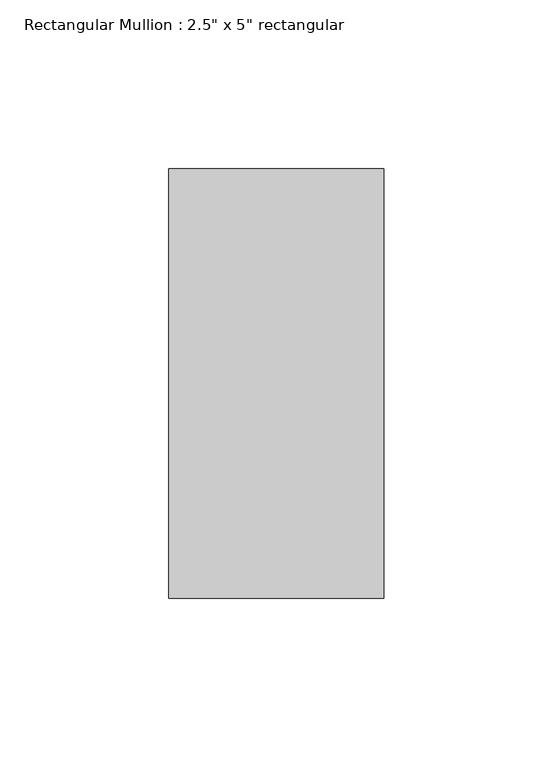
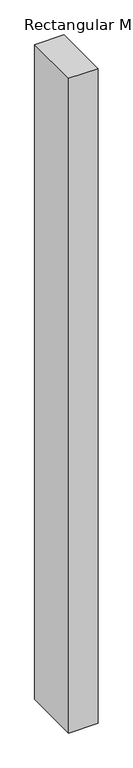
"""IFC4 building model written with IfcOpenShell, lengths in millimetres: member geometry."""

from ifc_helpers import new_model, si_unit, frame, origin, place, context, project, spatial, polyline, outline, extrude, source, transform, mapped, element, save


def member_d485efb4(model_context):
    return source(origin(), model_context, "Body", "SweptSolid", [
        extrude(outline(polyline([(0.0, 63.5), (0.0, -63.5), (-63.5, -63.5), (-63.5, 63.5), (0.0, 63.5)])), frame((0.0, 0.0, -1495.5694058), z_axis=(0.0, 0.0, 1.0), x_axis=(1.0, 0.0, 0.0)), (0.0, 0.0, 1.0), 1495.5694058),
    ])


if __name__ == "__main__":
    model = new_model("IFC4")
    model_context = context("Model", 3, world=origin())
    ifc_project = project(units=[si_unit("LENGTHUNIT", "METRE", prefix="MILLI")], contexts=[model_context])
    site = spatial("IfcSite", under=ifc_project)
    building = spatial("IfcBuilding", under=site)
    placement = place(None, origin())
    member_shape = member_d485efb4(model_context)
    element("IfcMember", 1, ObjectType="Rectangular Mullion : 2.5\" x 5\" rectangular", at=placement, inside=building, context=model_context, shape_type="MappedRepresentation", body=[
        mapped(member_shape, transform((0.0, 0.0, 0.0), x_axis=(1.0, 0.0, 0.0), y_axis=(0.0, 1.0, 0.0), z_axis=(0.0, 0.0, 1.0))),
    ])
    save(model, "model.ifc")

# Revit data of these elements
# Type "Rectangular Mullion : 2.5\" x 5\" rectangular"
#   built-in parameter 1007304 = 0.416667 (stored number, unit not read)
#   built-in parameter 1007301 = 0.104167 (stored number, unit not read)
#   built-in parameter 1007300 = 0.104167 (stored number, unit not read)
# Element 1 (IfcMember, "Rectangular Mullion : 2.5\" x 5\" rectangular")
#   Materials on its faces: "Aluminum"
# Materials
#   "Aluminum": class "Metal", colour RGB 247 247 247, transparency 0, Description = "Aluminum 6061", Cost = 0
